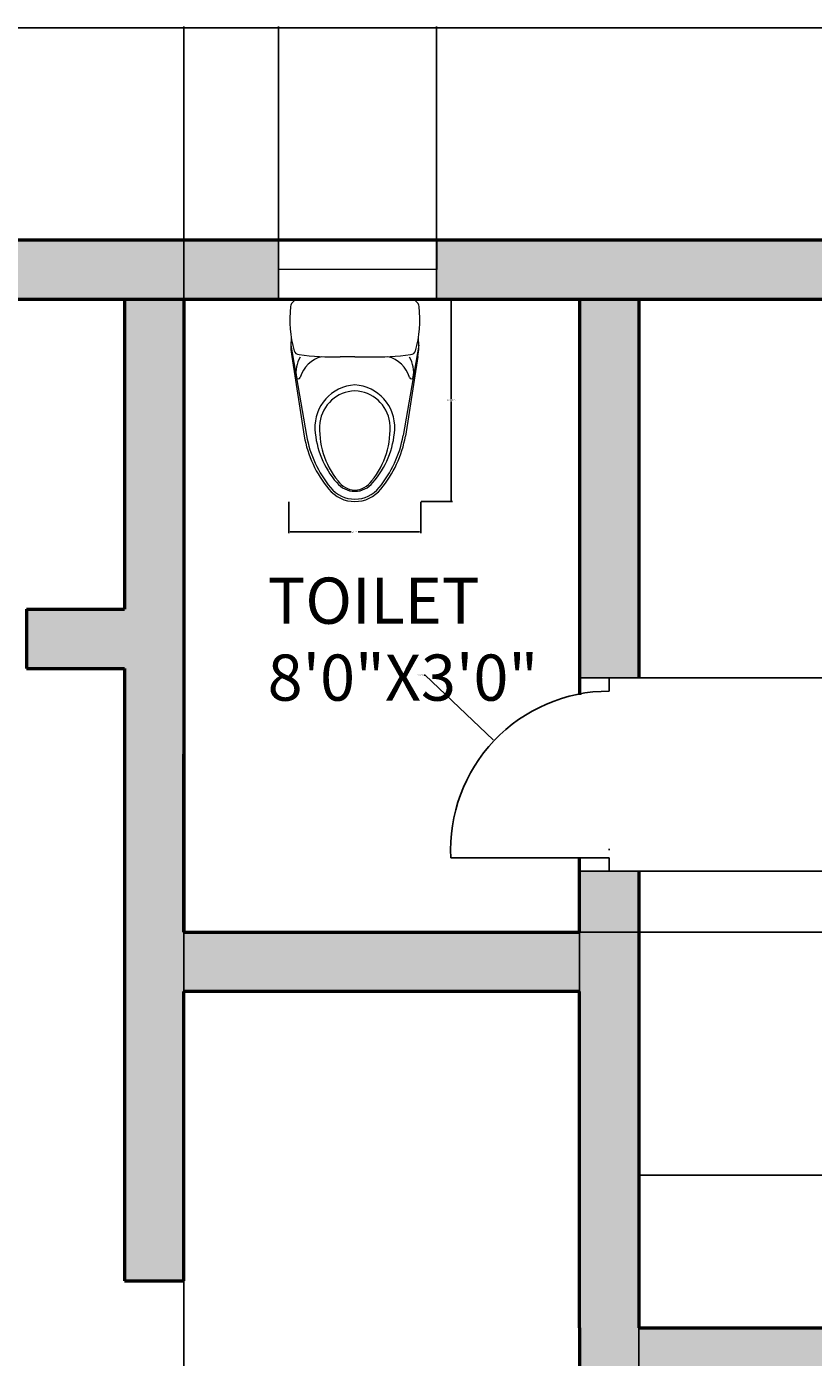
# Model space of a CAD drawing. Units: inches. Extents: x 1676 to 2199, y 1657 to 2783.
# Tile 8 of 10: x 1907 to 2027, y 2172 to 2373. Entities that reach past the tile are written whole.
import ezdxf

# ---------------------------------------------------------------- set-up
doc = ezdxf.new("R2010")
doc.units = ezdxf.units.IN
for name, color, linetype, lineweight in [('A-ANNO-DIMS', 2, 'Continuous', 18), ('A-AREA-IDEN', 7, 'Continuous', 18), ('A-DOOR', 4, 'Continuous', 25), ('A-FLOR-FIXT', 9, 'Continuous', 18), ('A-GLAZ', 4, 'Continuous', 18), ('A-WALL', 7, 'Continuous', 50)]:
    doc.layers.add(name, color=color, linetype=linetype, lineweight=lineweight)
doc.layers.add('A-WALL-PATT', color=251, linetype='Continuous', lineweight=13, true_color=0x636466)
doc.styles.get("Standard").update_dxf_attribs({"font": 'arial.ttf'})
doc.dimstyles.get("Standard").update_dxf_attribs({"dimtxt": 0.18, "dimasz": 0.18, "dimexe": 0.18, "dimexo": 0.0625, "dimgap": 0.09, "dimtad": 0, "dimtih": 1, "dimtoh": 1, "dimdec": 4, "dimzin": 0, "dimdsep": 46, "dimtxsty": 'Standard', "dimcen": 0.09, "dimadec": 0, "dimazin": 0, "dimtfac": 1, "dimtdec": 4, "dimtofl": 0, "dimtmove": 0, "dimatfit": 3, "dimfxl": 1, "dimtolj": 1, "dimtzin": 0, "dimarcsym": 0})

# ---------------------------------------------------------------- blocks, each defined once
blk = doc.blocks.new('A$C188A4A68')
at = {"ltscale": 20}
for p, q in [((0.2444, 0.7693), (0.0344, 0.7693)), ((0.2444, 0.7693), (0.4544, 0.7693)), ((0.0013, 0.5938), (0.0607, 0.2504)), ((0.4874, 0.5938), (0.428, 0.2504)), ((0.0054, 0.5515), (0.0519, 0.2489)), ((0.2444, 0.5498), (0.1889, 0.5498)), ((0.2444, 0.5498), (0.2998, 0.5498)), ((0.4833, 0.5515), (0.4368, 0.2489))]:
    blk.add_line(p, q, dxfattribs=at)
for centre, radius, start, end in [((0.0344, 0.7343), 0.0349, 90, 169.5926), ((0.4544, 0.7343), 0.0349, 10.4074, 90), ((0.442, 0.6914), 0.4447, 173.6395, 195.464), ((0.0467, 0.6914), 0.4447, 344.536, 6.3605), ((0.2125, 0.5932), 0.2113, 172.6498, 191.3659), ((0.2762, 0.5932), 0.2113, 348.6341, 7.3502), ((0.0333, 0.5802), 0.0213, 200.243, 267.1503), ((0.1632, 1.4554), 0.906, 261.6902, 271.6258), ((0.3255, 1.4554), 0.906, 268.3742, 278.3098), ((0.4554, 0.5802), 0.0213, 272.8497, 339.757), ((0.1303, 0.4913), 0.1097, 148.5069, 190.0488), ((0.1461, 0.4405), 0.1134, 104.1041, 164.1501), ((0.3426, 0.4405), 0.1134, 15.8499, 75.8959), ((0.3584, 0.4913), 0.1097, 349.9512, 31.4931), ((0.0297, 0.4734), 0.0075, 189.8264, 345.0875), ((0.459, 0.4734), 0.0075, 194.9125, 350.1736), ((0.254, 0.2824), 0.1613, 93.4333, 183.0038), ((0.2493, 0.2813), 0.1393, 92.0329, 172.0373), ((0.2347, 0.2824), 0.1613, 356.9962, 86.5667), ((0.2394, 0.2813), 0.1393, 7.9627, 87.9671), ((0.4311, 0.2946), 0.3389, 183.5042, 221.0229), ((0.4211, 0.2752), 0.3108, 175.3213, 219.2477), ((0.0676, 0.2752), 0.3108, 320.7523, 4.6787), ((0.0576, 0.2946), 0.3389, 318.9771, 356.4958), ((0.4781, 0.3243), 0.4328, 190.0297, 219.7428), ((0.4781, 0.3243), 0.4238, 190.0435, 219.7538), ((0.0106, 0.3243), 0.4238, 320.2462, 349.9565), ((0.0106, 0.3243), 0.4328, 320.2572, 349.9703), ((0.2444, 0.127), 0.118, 218.6774, 270), ((0.2444, 0.127), 0.088, 218.504, 270), ((0.2498, 0.1282), 0.0854, 215.5685, 266.3197), ((0.2389, 0.1282), 0.0854, 273.6803, 324.4315), ((0.2444, 0.127), 0.088, 270, 321.496), ((0.2444, 0.127), 0.118, 270, 321.3226), ((0.2444, 0.127), 0.127, 218.716, 270), ((0.2444, 0.127), 0.127, 270, 321.284)]:
    blk.add_arc(centre, radius, start, end, dxfattribs=at)
blk = doc.blocks.new('WIN-24')
for p, q in [((0, 0), (9, 0)), ((9, 0), (4.5, 0)), ((4.5, 0), (4.5, -24)), ((4.5, -24), (0, -24)), ((0, -24), (9, -24))]:
    blk.add_line(p, q)
blk = doc.blocks.new('*D13')
at = {"layer": 'A-ANNO-DIMS', "color": 0, "lineweight": -2, "transparency": 16777216}
for p, q in [((1967.08, 2332.09), (1971.8, 2332.09)), ((1971.62, 2331.91), (1971.62, 2316.92)), ((1971.62, 2301.57), (1971.62, 2316.55)), ((1967.08, 2301.39), (1971.8, 2301.39))]:
    blk.add_line(p, q, dxfattribs=at)
at = {"layer": 'A-ANNO-DIMS', "color": 0, "transparency": 16777216}
for points in [[(1971.59, 2331.91), (1971.65, 2331.91), (1971.62, 2332.09)], [(1971.59, 2301.57), (1971.65, 2301.57), (1971.62, 2301.39)]]:
    blk.add_solid(points, dxfattribs=at)
at = {"layer": 'Defpoints', "color": 0, "transparency": 16777216}
for p in [(1967.01, 2332.09), (1971.62, 2332.09), (1967.01, 2301.39)]:
    blk.add_point(p, dxfattribs=at)
at = {"layer": 'A-ANNO-DIMS', "color": 0, "transparency": 16777216, "insert": (1971.62, 2316.74), "char_height": 0.18, "attachment_point": 5}
blk.add_mtext('\\A1;WC 31 TYP.', dxfattribs=at)
blk = doc.blocks.new('*D14')
at = {"layer": 'A-ANNO-DIMS', "color": 0, "lineweight": -2, "transparency": 16777216}
for p, q in [((1947.01, 2301.33), (1947.01, 2296.6)), ((1967.01, 2301.33), (1967.01, 2296.6)), ((1947.19, 2296.78), (1956.48, 2296.78)), ((1966.83, 2296.78), (1957.54, 2296.78))]:
    blk.add_line(p, q, dxfattribs=at)
at = {"layer": 'A-ANNO-DIMS', "color": 0, "transparency": 16777216}
for points in [[(1947.19, 2296.81), (1947.19, 2296.75), (1947.01, 2296.78)], [(1966.83, 2296.81), (1966.83, 2296.75), (1967.01, 2296.78)]]:
    blk.add_solid(points, dxfattribs=at)
at = {"layer": 'Defpoints', "color": 0, "transparency": 16777216}
for p in [(1947.01, 2301.39), (1967.01, 2301.39), (1967.01, 2296.78)]:
    blk.add_point(p, dxfattribs=at)
at = {"layer": 'A-ANNO-DIMS', "color": 0, "transparency": 16777216, "insert": (1957.01, 2296.78), "char_height": 0.18, "attachment_point": 5}
blk.add_mtext('\\A1;20 TYP.', dxfattribs=at)
blk = doc.blocks.new('*D19')
at = {"layer": 'A-ANNO-DIMS', "color": 0, "lineweight": -2, "transparency": 16777216}
for p, q in [((1755.07, 2341.15), (1755.07, 2373.42)), ((1755.25, 2373.24), (1948.29, 2373.24)), ((2141.89, 2373.24), (1948.86, 2373.24)), ((2142.07, 2341.15), (2142.07, 2373.42))]:
    blk.add_line(p, q, dxfattribs=at)
at = {"layer": 'A-ANNO-DIMS', "color": 0, "transparency": 16777216}
for points in [[(1755.25, 2373.27), (1755.25, 2373.21), (1755.07, 2373.24)], [(2141.89, 2373.27), (2141.89, 2373.21), (2142.07, 2373.24)]]:
    blk.add_solid(points, dxfattribs=at)
at = {"layer": 'Defpoints', "color": 0, "transparency": 16777216}
for p in [(2142.07, 2373.24), (1755.07, 2341.09), (2142.07, 2341.09)]:
    blk.add_point(p, dxfattribs=at)
at = {"layer": 'A-ANNO-DIMS', "color": 0, "transparency": 16777216, "insert": (1948.57, 2373.24), "char_height": 0.18, "attachment_point": 5}
blk.add_mtext('\\A1;387', dxfattribs=at)
blk = doc.blocks.new('*D40')
at = {"layer": 'A-ANNO-DIMS', "color": 0, "lineweight": -2, "transparency": 16777216}
for p, q in [((1931.07, 2236.02), (1931.07, 1695.28)), ((1991.07, 2236.02), (1991.07, 1695.28)), ((1931.25, 1695.46), (1960.86, 1695.46)), ((1990.89, 1695.46), (1961.29, 1695.46))]:
    blk.add_line(p, q, dxfattribs=at)
at = {"layer": 'A-ANNO-DIMS', "color": 0, "transparency": 16777216}
for points in [[(1931.25, 1695.49), (1931.25, 1695.43), (1931.07, 1695.46)], [(1990.89, 1695.49), (1990.89, 1695.43), (1991.07, 1695.46)]]:
    blk.add_solid(points, dxfattribs=at)
at = {"layer": 'Defpoints', "color": 0, "transparency": 16777216}
for p in [(1931.07, 2236.09), (1991.07, 2236.09), (1991.07, 1695.46)]:
    blk.add_point(p, dxfattribs=at)
at = {"layer": 'A-ANNO-DIMS', "color": 0, "transparency": 16777216, "insert": (1961.07, 1695.46), "char_height": 0.18, "attachment_point": 5}
blk.add_mtext('\\A1;60', dxfattribs=at)
blk = doc.blocks.new('*D41')
at = {"layer": 'A-ANNO-DIMS', "color": 0, "lineweight": -2, "transparency": 16777216}
for p, q in [((1991.14, 2245.34), (2174.4, 2245.34)), ((2174.22, 2245.16), (2174.22, 2240.9)), ((2174.22, 2236.27), (2174.22, 2240.53)), ((1991.14, 2236.09), (2174.4, 2236.09))]:
    blk.add_line(p, q, dxfattribs=at)
at = {"layer": 'A-ANNO-DIMS', "color": 0, "transparency": 16777216}
for points in [[(2174.19, 2245.16), (2174.25, 2245.16), (2174.22, 2245.34)], [(2174.19, 2236.27), (2174.25, 2236.27), (2174.22, 2236.09)]]:
    blk.add_solid(points, dxfattribs=at)
at = {"layer": 'Defpoints', "color": 0, "transparency": 16777216}
for p in [(1991.07, 2245.34), (2174.22, 2245.34), (1991.07, 2236.09)]:
    blk.add_point(p, dxfattribs=at)
at = {"layer": 'A-ANNO-DIMS', "color": 0, "transparency": 16777216, "insert": (2174.22, 2240.71), "char_height": 0.18, "attachment_point": 5}
blk.add_mtext('\\A1;9.255', dxfattribs=at)
blk = doc.blocks.new('*D42')
at = {"layer": 'A-ANNO-DIMS', "color": 0, "lineweight": -2, "transparency": 16777216}
for p, q in [((1991.14, 2274.63), (2174.4, 2274.63)), ((2174.22, 2274.45), (2174.22, 2260.17)), ((2174.22, 2245.52), (2174.22, 2259.81)), ((1991.14, 2245.34), (2174.4, 2245.34))]:
    blk.add_line(p, q, dxfattribs=at)
at = {"layer": 'A-ANNO-DIMS', "color": 0, "transparency": 16777216}
for points in [[(2174.19, 2274.45), (2174.25, 2274.45), (2174.22, 2274.63)], [(2174.19, 2245.52), (2174.25, 2245.52), (2174.22, 2245.34)]]:
    blk.add_solid(points, dxfattribs=at)
at = {"layer": 'Defpoints', "color": 0, "transparency": 16777216}
for p in [(1991.07, 2274.63), (2174.22, 2274.63), (1991.07, 2245.34)]:
    blk.add_point(p, dxfattribs=at)
at = {"layer": 'A-ANNO-DIMS', "color": 0, "transparency": 16777216, "insert": (2174.22, 2259.99), "char_height": 0.18, "attachment_point": 5}
blk.add_mtext('\\A1;29.29', dxfattribs=at)
blk = doc.blocks.new('*D43')
at = {"layer": 'A-ANNO-DIMS', "color": 0, "lineweight": -2, "transparency": 16777216}
for p, q in [((1931.07, 2332.15), (1931.07, 2373.42)), ((1931.25, 2373.24), (1937.79, 2373.24)), ((1945.24, 2373.24), (1938.7, 2373.24)), ((1945.42, 2332.15), (1945.42, 2373.42))]:
    blk.add_line(p, q, dxfattribs=at)
at = {"layer": 'A-ANNO-DIMS', "color": 0, "transparency": 16777216}
for points in [[(1931.25, 2373.27), (1931.25, 2373.21), (1931.07, 2373.24)], [(1945.24, 2373.27), (1945.24, 2373.21), (1945.42, 2373.24)]]:
    blk.add_solid(points, dxfattribs=at)
at = {"layer": 'Defpoints', "color": 0, "transparency": 16777216}
for p in [(1945.42, 2373.24), (1931.07, 2332.09), (1945.42, 2332.09)]:
    blk.add_point(p, dxfattribs=at)
at = {"layer": 'A-ANNO-DIMS', "color": 0, "transparency": 16777216, "insert": (1938.25, 2373.24), "char_height": 0.18, "attachment_point": 5}
blk.add_mtext('\\A1;14.347', dxfattribs=at)
blk = doc.blocks.new('*D44')
at = {"layer": 'A-ANNO-DIMS', "color": 0, "lineweight": -2, "transparency": 16777216}
for p, q in [((1945.42, 2332.15), (1945.42, 2373.42)), ((1945.6, 2373.24), (1957.2, 2373.24)), ((1969.24, 2373.24), (1957.64, 2373.24)), ((1969.42, 2332.15), (1969.42, 2373.42))]:
    blk.add_line(p, q, dxfattribs=at)
at = {"layer": 'A-ANNO-DIMS', "color": 0, "transparency": 16777216}
for points in [[(1945.6, 2373.27), (1945.6, 2373.21), (1945.42, 2373.24)], [(1969.24, 2373.27), (1969.24, 2373.21), (1969.42, 2373.24)]]:
    blk.add_solid(points, dxfattribs=at)
at = {"layer": 'Defpoints', "color": 0, "transparency": 16777216}
for p in [(1969.42, 2373.24), (1945.42, 2332.09), (1969.42, 2332.09)]:
    blk.add_point(p, dxfattribs=at)
at = {"layer": 'A-ANNO-DIMS', "color": 0, "transparency": 16777216, "insert": (1957.42, 2373.24), "char_height": 0.18, "attachment_point": 5}
blk.add_mtext('\\A1;24', dxfattribs=at)
blk = doc.blocks.new('*D45')
at = {"layer": 'A-ANNO-DIMS', "color": 0, "lineweight": -2, "transparency": 16777216}
for p, q in [((2000.07, 2167.15), (2000.07, 2199.42)), ((2000.25, 2199.24), (2044.86, 2199.24)), ((2089.89, 2199.24), (2045.29, 2199.24)), ((2090.07, 2167.15), (2090.07, 2199.42))]:
    blk.add_line(p, q, dxfattribs=at)
at = {"layer": 'A-ANNO-DIMS', "color": 0, "transparency": 16777216}
for points in [[(2000.25, 2199.27), (2000.25, 2199.21), (2000.07, 2199.24)], [(2089.89, 2199.27), (2089.89, 2199.21), (2090.07, 2199.24)]]:
    blk.add_solid(points, dxfattribs=at)
at = {"layer": 'Defpoints', "color": 0, "transparency": 16777216}
for p in [(2090.07, 2199.24), (2000.07, 2167.09), (2090.07, 2167.09)]:
    blk.add_point(p, dxfattribs=at)
at = {"layer": 'A-ANNO-DIMS', "color": 0, "transparency": 16777216, "insert": (2045.07, 2199.24), "char_height": 0.18, "attachment_point": 5}
blk.add_mtext('\\A1;90', dxfattribs=at)
blk = doc.blocks.new('*D78')
at = {"layer": 'A-ANNO-DIMS', "color": 0, "lineweight": -2, "transparency": 16777216}
for p, q in [((1967.5, 2275.07), (1967.68, 2275.07)), ((1967.68, 2275.07), (1978.01, 2265.27)), ((1995.48, 2248.6), (1995.66, 2248.6)), ((1995.57, 2248.51), (1995.57, 2248.69))]:
    blk.add_line(p, q, dxfattribs=at)
at = {"layer": 'A-ANNO-DIMS', "color": 0, "transparency": 16777216}
blk.add_solid([(1978.03, 2265.29), (1977.99, 2265.25), (1978.14, 2265.14)], dxfattribs=at)
at = {"layer": 'Defpoints', "color": 0, "transparency": 16777216}
for p in [(1978.14, 2265.14), (1995.57, 2248.6)]:
    blk.add_point(p, dxfattribs=at)
at = {"layer": 'A-ANNO-DIMS', "color": 0, "transparency": 16777216, "insert": (1966.95, 2275.07), "char_height": 0.18, "attachment_point": 5}
blk.add_mtext('\\A1;R24.033', dxfattribs=at)

msp = doc.modelspace()

# ---------------------------------------------------------------- hatches: boundary and pattern name
at = {"layer": 'A-WALL-PATT'}
h = msp.add_hatch(color=256, dxfattribs=at)
h.dxf.hatch_style = 1
h.paths.add_polyline_path([(1945.4216, 2336.5871), (1945.4216, 2341.0871), (1755.075, 2341.0871), (1755.075, 2323.0739), (1764.075, 2323.0739), (1764.075, 2332.0871), (1945.4216, 2332.0871)])
h.paths.add_polyline_path([(1764.075, 2299.0739), (1755.075, 2299.0739), (1755.075, 2266.2601), (1759.575, 2266.2601), (1764.075, 2266.2601)])
h.paths.add_polyline_path([(1843.075, 2285.0871), (1764.075, 2285.0871), (1764.075, 2276.0871), (1843.075, 2276.0871)])
h.paths.add_polyline_path([(1931.075, 2332.0871), (1922.075, 2332.0871), (1922.075, 2285.0871), (1907.247, 2285.0871), (1907.247, 2276.0871), (1922.075, 2276.0871), (1922.075, 2263.0871), (1922.075, 2214.434), (1922.075, 2183.2198), (1931.075, 2183.2198), (1931.075, 2214.434), (1931.075, 2227.0871), (1991.075, 2227.0871), (1991.075, 2176.0871), (1991.075, 2167.0871), (2000.075, 2167.0871), (2133.075, 2167.0871), (2133.075, 2176.0871), (2000.075, 2176.0871), (2000.075, 2245.3418), (1995.575, 2245.3418), (1991.075, 2245.3418), (1991.075, 2236.0871), (1931.075, 2236.0871)])
h.paths.add_polyline_path([(2000.075, 2332.0871), (1991.075, 2332.0871), (1991.075, 2285.0871), (1991.075, 2274.6339), (2000.075, 2274.6339), (2000.075, 2285.0871)], flags=17)
h.paths.add_polyline_path([(2142.075, 2341.0871), (1969.4216, 2341.0871), (1969.4216, 2332.0871), (2133.075, 2332.0871), (2133.075, 2298.2101), (2142.075, 2298.2101)])
h.paths.add_polyline_path([(2142.075, 1844.9908), (2133.075, 1844.9908), (2133.075, 1790.0871), (2061.2106, 1790.0871), (2061.2106, 1781.0871), (2142.075, 1781.0871)])
h.paths.add_polyline_path([(2001.2106, 1790.0871), (1966.075, 1790.0871), (1966.075, 1957.0871), (1973.4183, 1957.0871), (1973.4183, 1966.0871), (1966.075, 1966.0871), (1966.075, 1983.1515), (1957.075, 1983.1515), (1957.075, 1899.0871), (1946.8789, 1899.0871), (1946.8789, 1890.0871), (1957.075, 1890.0871), (1957.075, 1781.0871), (2001.2106, 1781.0871), (2001.2106, 1785.5871)])
h.paths.add_polyline_path([(1876.3163, 1894.5871), (1876.3163, 1899.0871), (1820.9237, 1899.0871), (1820.9237, 1890.0871), (1876.3163, 1890.0871)])
h.paths.add_polyline_path([(1764.075, 2093.9207), (1759.575, 2093.9207), (1755.075, 2093.9207), (1755.075, 2019.5723), (1764.075, 2019.5723)])
h.paths.add_polyline_path([(1878.3926, 2083.0871), (1764.075, 2083.0871), (1764.075, 2074.0871), (1878.3926, 2074.0871)])
h.paths.add_polyline_path([(1764.075, 1959.5723), (1755.075, 1959.5723), (1755.075, 1890.0871), (1784.9237, 1890.0871), (1784.9237, 1894.5871), (1784.9237, 1899.0871), (1764.075, 1899.0871)])
h.paths.add_polyline_path([(2133.075, 2047.0871), (2000.075, 2047.0871), (1966.075, 2047.0871), (1957.075, 2047.0871), (1938.4046, 2047.0871), (1938.4046, 2038.0871), (1957.075, 2038.0871), (1957.075, 2026.1604), (1966.075, 2026.1604), (1966.075, 2038.0871), (2039.075, 2038.0871), (2039.075, 2011.4216), (2048.075, 2011.4216), (2048.075, 2038.0871), (2133.075, 2038.0871)])
h.paths.add_polyline_path([(2133.075, 1966.0871), (2048.075, 1966.0871), (2048.075, 1972.5045), (2039.075, 1972.5045), (2039.075, 1966.0871), (2025.1075, 1966.0871), (2025.1075, 1957.0871), (2133.075, 1957.0871)])
h.paths.add_polyline_path([(1764.075, 2206.2601), (1755.075, 2206.2601), (1755.075, 2153.9207), (1764.075, 2153.9207)])

# ---------------------------------------------------------------- linework, layer by layer
at = {"layer": 'A-DOOR'}
for p, q in [((1991.075, 2274.6339), (2000.075, 2274.6339)), ((2000.075, 2274.6339), (1995.575, 2274.6339)), ((1995.575, 2274.6339), (1995.575, 2272.6339)), ((1995.575, 2247.3418), (1971.575, 2247.3418)), ((1995.575, 2245.3418), (1995.575, 2247.3418)), ((1991.075, 2245.3418), (2000.075, 2245.3418)), ((2000.075, 2245.3418), (1995.575, 2245.3418))]:
    msp.add_line(p, q, dxfattribs=at)
msp.add_arc((1995.575, 2248.6009), 24.033, 90, 183.003225, dxfattribs=at)
at = {"layer": 'A-WALL'}
for p, q in [((1755.075, 2341.0871), (2142.075, 2341.0871)), ((1764.075, 2332.0871), (2133.075, 2332.0871)), ((1922.075, 2332.0871), (1922.075, 2285.0871)), ((1931.075, 2332.0871), (1931.075, 2285.0871)), ((1931.075, 2332.0871), (1931.075, 2236.0871)), ((1991.075, 2332.0871), (1991.075, 2285.0871)), ((2000.075, 2332.0871), (2000.075, 2285.0871)), ((1907.247, 2285.0871), (1907.247, 2276.0871)), ((1907.247, 2285.0871), (1922.075, 2285.0871)), ((1931.075, 2285.0871), (1931.075, 2272.0871)), ((1991.075, 2285.0871), (1991.075, 2272.0871)), ((2000.075, 2285.0871), (2000.075, 2274.6339)), ((1907.247, 2276.0871), (1922.075, 2276.0871)), ((1922.075, 2276.0871), (1922.075, 2263.0871)), ((1922.075, 2263.0871), (1922.075, 2214.434)), ((1931.075, 2236.0871), (1931.075, 2263.0871)), ((1991.075, 2236.0871), (1991.075, 2247.3418)), ((2000.075, 2245.3418), (2000.075, 2176.0871)), ((1931.075, 2236.0871), (1991.075, 2236.0871)), ((2000.075, 2236.0871), (2000.075, 2227.0871)), ((1931.075, 2214.434), (1931.075, 2227.0871)), ((1991.075, 2227.0871), (1931.075, 2227.0871)), ((1991.075, 2176.0871), (1991.075, 2227.0871)), ((1922.075, 2214.434), (1922.075, 2183.2198)), ((1931.075, 2183.2198), (1931.075, 2214.434)), ((1922.075, 2183.2198), (1931.075, 2183.2198)), ((1991.075, 2176.0871), (1991.075, 2167.0871)), ((2000.075, 2176.0871), (2133.075, 2176.0871))]:
    msp.add_line(p, q, dxfattribs=at)

# ---------------------------------------------------------------- block references
at = {"layer": 'A-FLOR-FIXT', "xscale": 39.90803308922938, "yscale": 39.90803308922938, "zscale": 39.90803308922938}
msp.add_blockref('A$C188A4A68', (1947.2603, 2301.3876), dxfattribs=at)
at = {"layer": 'A-GLAZ', "extrusion": (0, 0, -1), "zscale": -1, "rotation": 90}
msp.add_blockref('WIN-24', (-1969.4216, 2332.0871), dxfattribs=at)

# ---------------------------------------------------------------- texts
at = {"layer": 'A-AREA-IDEN', "insert": (1943.7904, 2289.8528), "char_height": 7, "attachment_point": 1}
msp.add_mtext_dynamic_manual_height_columns('TOILET\\P8\'0"X3\'0"', width=71.901711, gutter_width=12.5, heights=[0], dxfattribs=at)

# ---------------------------------------------------------------- dimensions: what is measured, and where the dimension line sits
at = {"layer": 'A-ANNO-DIMS'}
for base, p1, p2, override, picture, middle in [((2142.075, 2373.2371), (1755.075, 2341.0871), (2142.075, 2341.0871), {"dimdec": 0, "dimlfac": 1, "dimrnd": 0, "dimzin": 0, "dimdsep": 46, "dimlunit": 2}, '*D19', (1948.575, 2373.2371)), ((1945.4216, 2373.2371), (1931.075, 2332.0871), (1945.4216, 2332.0871), {"dimdec": 3, "dimlfac": 1, "dimrnd": 0, "dimzin": 0, "dimdsep": 46, "dimlunit": 2}, '*D43', (1938.2483, 2373.2371)), ((1969.4216, 2373.2371), (1945.4216, 2332.0871), (1969.4216, 2332.0871), {"dimdec": 0, "dimlfac": 1, "dimrnd": 0, "dimzin": 0, "dimdsep": 46, "dimlunit": 2}, '*D44', (1957.4216, 2373.2371)), ((1991.075, 1695.4613), (1931.075, 2236.0871), (1991.075, 2236.0871), {"dimdec": 0, "dimlfac": 1, "dimrnd": 0, "dimzin": 0, "dimdsep": 46, "dimlunit": 2}, '*D40', (1961.075, 1695.4613))]:
    dim = msp.add_linear_dim(base=base, p1=p1, p2=p2, dimstyle='Standard', override=override, dxfattribs=at)
    dim.commit()
    dim.dimension.update_dxf_attribs({"geometry": picture, "text_midpoint": middle})
dim = msp.add_linear_dim(base=(1971.6187, 2332.0871), p1=(1967.0137, 2301.3876), p2=(1967.0137, 2332.0871), angle=90, text='WC <> TYP.', dimstyle='Standard', override={"dimdec": 0, "dimlfac": 1, "dimrnd": 0, "dimzin": 0, "dimdsep": 46, "dimlunit": 2}, dxfattribs=at)
dim.commit()
dim.dimension.update_dxf_attribs({"geometry": '*D13', "text_midpoint": (1971.6187, 2316.7373)})
dim = msp.add_linear_dim(base=(1967.0137, 2296.7827), p1=(1947.0099, 2301.3876), p2=(1967.0137, 2301.3876), text='<> TYP.', dimstyle='Standard', override={"dimdec": 0, "dimlfac": 1, "dimrnd": 0, "dimzin": 0, "dimdsep": 46, "dimlunit": 2}, dxfattribs=at)
dim.commit()
dim.dimension.update_dxf_attribs({"geometry": '*D14', "text_midpoint": (1957.0118, 2296.7827)})
dim = msp.add_radius_dim(center=(1995.575, 2248.6009), mpoint=(1978.142, 2265.144), dimstyle='Standard', override={"dimdec": 3, "dimlfac": 1, "dimrnd": 0, "dimzin": 0, "dimdsep": 46, "dimlunit": 2}, dxfattribs=at)
dim.commit()
dim.dimension.update_dxf_attribs({"geometry": '*D78', "text_midpoint": (1966.9524, 2275.0699), "dimtype": 164})
for base, p1, p2, angle, override, picture, middle in [((2174.225, 2274.6339), (1991.075, 2245.3418), (1991.075, 2274.6339), 90, {"dimdec": 2, "dimlfac": 1, "dimrnd": 0, "dimzin": 0, "dimdsep": 46, "dimlunit": 2}, '*D42', (2174.225, 2259.9878)), ((2174.225, 2245.3418), (1991.075, 2236.0871), (1991.075, 2245.3418), 90, {"dimdec": 3, "dimlfac": 1, "dimrnd": 0, "dimzin": 0, "dimdsep": 46, "dimlunit": 2}, '*D41', (2174.225, 2240.7144)), ((2090.075, 2199.2371), (2000.075, 2167.0871), (2090.075, 2167.0871), 0, {"dimdec": 0, "dimlfac": 1, "dimrnd": 0, "dimzin": 0, "dimdsep": 46, "dimlunit": 2}, '*D45', (2045.075, 2199.2371))]:
    dim = msp.add_linear_dim(base=base, p1=p1, p2=p2, angle=angle, dimstyle='Standard', override=override, dxfattribs=at)
    dim.commit()
    dim.dimension.update_dxf_attribs({"geometry": picture, "text_midpoint": middle})

doc.saveas('drawing.dxf')
